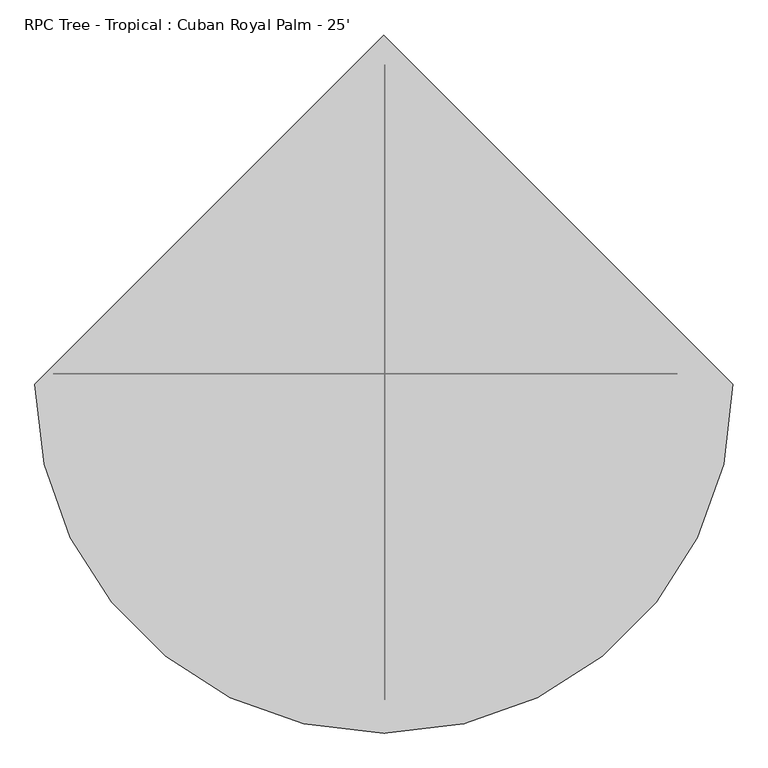
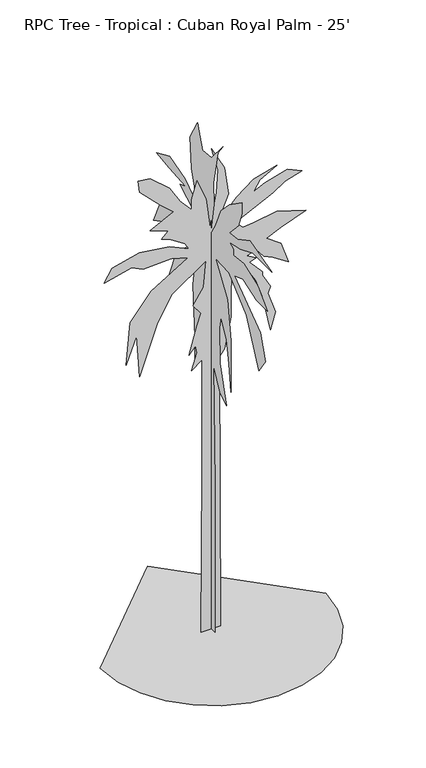
"""IFC4 building model written with IfcOpenShell, lengths in millimetres: geographic element geometry, RPC Tree - Tropical : Cuban Royal Palm - 25'."""

from ifc_helpers import new_model, si_unit, origin, place, context, project, spatial, triangles, source, transform, mapped, element, save


def rpc_tree_tropical_cuban_royal_palm_25_6f0ceb55(model_context):
    return source(origin(), model_context, "Body", "Tessellation", [
        triangles([(-54.3826135, -0.017491, 0.0009437), (-150.0419681, -0.0174994, 0.0009479), (-130.9099418, -0.0179382, 2494.6483109), (-130.9096875, -0.0182426, 4197.3711227), (-283.9640988, -0.0182154, 4082.5885941), (-207.4377743, -0.0182632, 4331.3053894), (-226.5690375, -0.0182829, 4446.0876274), (-322.2291687, -0.0182582, 4331.3053894), (-207.4375199, -0.0183385, 4752.2081863), (-150.0417137, -0.0183718, 4924.3947693), (-264.8328356, -0.0183942, 5077.4551941), (-111.778179, -0.0184419, 5307.0196701), (-73.5143854, -0.0185154, 5708.7968903), (-570.9431663, -0.0184321, 5364.4237244), (-781.3921303, -0.0183579, 5000.9249817), (-1049.2399527, -0.0182128, 4254.775177), (-1087.5024427, -0.0183274, 4905.2686111), (-1240.5575626, -0.0182489, 4503.4916817), (-1183.1638275, -0.0183643, 5134.8336685), (-877.0535151, -0.0184461, 5517.4841492), (-341.3604137, -0.0185277, 5842.7305756), (-590.0744476, -0.0185305, 5919.260788), (-991.8436014, -0.0185095, 5900.10905), (-1164.030039, -0.0185156, 5976.6392624), (-1565.7991928, -0.018481, 5880.9828918), (-1451.0091064, -0.0185202, 6072.2956329), (-1049.2399527, -0.0185549, 6167.9775833), (-609.2056927, -0.0185639, 6110.5735291), (-322.2291687, -0.0185524, 5976.6392624), (-379.6254836, -0.018567, 6072.2956329), (-609.2056927, -0.0185844, 6225.3560577), (-723.9983225, -0.0185862, 6263.6339539), (-628.3394812, -0.0186075, 6359.2903244), (-896.1847601, -0.0186129, 6454.9461136), (-551.8119212, -0.0186587, 6627.1326965), (-743.1295675, -0.0186811, 6799.3192795), (-1049.2399527, -0.0187225, 7105.4395477), (-1068.3711977, -0.0187524, 7277.6261307), (-896.1847601, -0.0187566, 7258.4743927), (-609.2056927, -0.0187246, 7009.7581787), (-456.1505364, -0.0186868, 6761.0413834), (-283.9640988, -0.0186602, 6569.7286423), (-283.9640988, -0.0186875, 6722.7890671), (-207.4375199, -0.0187388, 6990.6320206), (-73.5143854, -0.0186865, 6665.3850128), (-16.1188494, -0.0186069, 6206.2298996), (79.5405301, -0.0187, 6703.6629089), (98.6725473, -0.0187624, 7048.0354935), (3.0131737, -0.0188232, 7411.5348175), (194.3319064, -0.0187666, 7048.0354935), (251.7277126, -0.0186938, 6627.1326965), (79.5405301, -0.018611, 6206.2298996), (366.5190888, -0.0186818, 6531.476326), (615.2330864, -0.0187268, 6722.7890671), (959.6059616, -0.018759, 6818.4454376), (710.8919277, -0.0187242, 6684.5367508), (615.2330864, -0.0186926, 6531.476326), (787.419524, -0.0187138, 6608.0065384), (1112.6611542, -0.0187452, 6703.6629089), (1323.1125526, -0.0187373, 6608.0065384), (1074.3985914, -0.0187127, 6531.476326), (902.2121538, -0.0186847, 6416.6687988), (347.3878438, -0.0186125, 6148.8258453), (462.1779302, -0.018597, 6034.0433167), (615.2330864, -0.0186071, 6053.1694748), (959.6059616, -0.0186324, 6110.5735291), (1380.5089039, -0.0186269, 5976.6392624), (1017.0023129, -0.018587, 5842.7305756), (806.550769, -0.0185607, 5747.074205), (1017.0023129, -0.0185426, 5594.0143616), (1131.7923992, -0.0184894, 5268.7673538), (902.2121538, -0.0185068, 5421.8277786), (768.288279, -0.0185112, 5479.2062531), (615.2330864, -0.0185387, 5670.544574), (615.2330864, -0.0185284, 5613.1405197), (519.5742451, -0.0185174, 5574.8882034), (653.4956491, -0.0185096, 5498.357991), (557.8367715, -0.0184985, 5460.0800949), (749.1570339, -0.0184693, 5249.6411957), (749.1570339, -0.018459, 5192.2371414), (863.9471203, -0.0184264, 4981.7988235), (825.6846302, -0.0184076, 4886.142453), (940.4747166, -0.0183545, 4560.8957359), (863.9471203, -0.0183067, 4312.1792313), (749.1570339, -0.0184009, 4866.990715), (653.4956491, -0.018448, 5153.9848251), (481.3092115, -0.0184918, 5440.9539368), (309.1227739, -0.0184979, 5517.4841492), (289.9915107, -0.0184287, 5134.8336685), (289.9915107, -0.0183534, 4713.9558701), (194.3319064, -0.0182671, 4254.775177), (117.8043192, -0.0182467, 4159.1188065), (136.9360911, -0.0175052, 0.0009354), (-0.003708, 89.5986644, 0.000495), (-0.0037084, 163.6334895, 0.0005082), (-0.003708, 163.6334895, 1826.7789024), (-0.003706, 145.1250443, 4288.4300995), (-0.0037076, 219.1593699, 4177.3813545), (-0.0037057, 404.2456741, 3788.6856033), (-0.0037071, 404.2456741, 4251.4224747), (-0.0037068, 459.7725537, 5028.7883972), (-0.0037083, 385.7367022, 5565.5410995), (-0.0037091, 533.8058619, 5398.9425476), (-0.0037068, 792.9287807, 4862.190136), (-0.0037064, 1089.0671001, 4492.0362762), (-0.0037084, 1311.1695316, 4140.3737297), (-0.0037071, 1052.0491562, 4843.6988228), (-0.0037074, 885.4710245, 5250.8858871), (-0.0037074, 515.2968899, 5621.065036), (-0.003709, 681.8750216, 5584.0318314), (-0.0037073, 903.9799965, 5565.5410995), (-0.0037076, 1107.5760721, 5602.5487244), (-0.0037076, 1459.2413074, 5417.4588593), (-0.0037087, 1274.1542038, 5824.6462143), (-0.0037067, 1070.5581282, 5824.6462143), (-0.0037071, 996.5223129, 6139.3008453), (-0.0037076, 644.859621, 6065.2600159), (-0.0037089, 422.7546461, 6176.3084702), (-0.0037091, 792.9287807, 6379.9146469), (-0.0037059, 644.859621, 6435.4391647), (-0.0037081, 1052.0491562, 6472.4467896), (-0.0037064, 1385.2054195, 6509.4799942), (-0.0037073, 1052.0491562, 6657.5366547), (-0.0037075, 663.368593, 6546.487619), (-0.0037092, 348.7187945, 6324.3907104), (-0.003707, 496.7904977, 6805.6183136), (-0.0037068, 533.8058619, 7268.3296051), (-0.0037076, 348.7187945, 7601.4755493), (-0.0037068, 311.703394, 7490.427095), (-0.0037069, 219.1593699, 7249.8132935), (-0.0037086, -2.9445681, 7268.3296051), (-0.0037062, -299.0821622, 7619.9924423), (-0.0037078, -169.5227376, 7453.4194702), (-0.0037084, -58.4704863, 6916.6673492), (-0.0037085, -76.9791948, 6602.0121368), (-0.003709, 15.5640629, 6083.7763275), (-0.0037058, -113.9968663, 6287.3575058), (-0.0037085, -243.5573174, 6602.0121368), (-0.0037085, -465.6602757, 6824.1096268), (-0.003709, -780.3075308, 7046.2321152), (-0.003709, -780.3075308, 6879.6341446), (-0.0037083, -687.765287, 6639.0453415), (-0.0037091, -465.6602757, 6398.4315399), (-0.0037063, -669.256315, 6416.9228531), (-0.0037092, -983.9036064, 6583.4958252), (-0.0037074, -1539.164772, 6435.4391647), (-0.0037081, -1057.9394217, 6435.4391647), (-0.0037072, -743.2921303, 6305.8738174), (-0.0037083, -465.6602757, 6250.3492996), (-0.0037076, -558.2050993, 6194.8253632), (-0.003708, -558.2050993, 6102.2932205), (-0.0037077, -835.8344467, 6139.3008453), (-0.0037071, -1187.4996094, 6009.735498), (-0.0037064, -1428.1110855, 5769.1216965), (-0.0037087, -1150.4816654, 5769.1216965), (-0.0037066, -798.8165028, 5880.1701508), (-0.0037081, -595.2230069, 5806.1549011), (-0.0037069, -1243.0264526, 5324.9267166), (-0.0037071, -1372.586713, 4954.7475677), (-0.0037067, -1206.0085814, 4714.1337662), (-0.0037072, -891.36129, 5380.4512344), (-0.0037069, -447.1538472, 5769.1216965), (-0.003706, -113.9968663, 5787.6380081), (-0.0037066, -410.1359396, 5324.9267166), (-0.0037068, -502.6781834, 4751.141391), (-0.0037091, -502.6781834, 3955.2841553), (-0.0037069, -447.1538472, 4362.470929), (-0.003708, -391.6269676, 4695.6171638), (-0.0037083, -243.5573174, 4954.7475677), (-0.0037075, -206.5399003, 4769.6579933), (-0.0037065, -225.0485998, 4232.9058723), (-0.0037092, -391.6269676, 3677.6368584), (-0.0037079, -225.0485998, 3788.6856033), (-0.0037085, -58.4704863, 4103.3405251), (-0.0037063, -95.4881577, 2289.4952808), (-0.0037089, -95.4881577, 0.0004619), (-1653.0963352, -49.1291369, 0.0005424), (-1609.512513, -426.8745255, 0.000473), (-1485.3879673, -773.7746447, 0.0004055), (-1290.6616264, -1079.890044, 0.0003423), (-1035.2724913, -1335.2792519, 0.0002854), (-729.1570919, -1530.0055927, 0.0002372), (-382.2594435, -1654.1301384, 0.0001999), (-4.5121786, -1697.7139606, 0.0001756), (373.234849, -1654.1301384, 0.0001668), (720.1324247, -1530.0055927, 0.0001739), (1026.2478968, -1335.2792519, 0.0001953), (1281.6370319, -1079.890044, 0.0002298), (1476.3633728, -773.7746447, 0.000276), (1600.4879185, -426.8745255, 0.0003326), (1644.0717407, -49.1291369, 0.0003983), (-4.5124832, 1599.4541153, 0.0003027)], [[54, 55, 56], [48, 49, 50], [17, 18, 19], [15, 16, 17], [7, 8, 9], [83, 84, 85], [82, 83, 85], [4, 5, 6], [70, 71, 72], [66, 67, 68], [43, 44, 45], [59, 60, 61], [24, 25, 26], [24, 26, 27], [33, 34, 35], [76, 77, 78], [58, 59, 61], [58, 61, 62], [31, 32, 33], [42, 43, 45], [42, 45, 46], [37, 38, 39], [54, 56, 57], [53, 54, 57], [23, 24, 27], [23, 27, 28], [22, 23, 28], [22, 28, 29], [21, 22, 29], [58, 62, 63], [57, 58, 63], [53, 57, 63], [52, 53, 63], [36, 37, 39], [36, 39, 40], [36, 40, 41], [35, 36, 41], [35, 41, 42], [69, 70, 72], [69, 72, 73], [69, 73, 74], [65, 66, 68], [65, 68, 69], [65, 69, 74], [64, 65, 74], [47, 48, 50], [47, 50, 51], [46, 47, 51], [46, 51, 52], [33, 35, 42], [82, 85, 86], [81, 82, 86], [80, 81, 86], [33, 42, 46], [31, 33, 46], [30, 31, 46], [29, 30, 46], [15, 17, 19], [15, 19, 20], [14, 15, 20], [14, 20, 21], [13, 14, 21], [92, 93, 1], [92, 1, 2], [92, 2, 3], [92, 3, 4], [80, 86, 87], [79, 80, 87], [78, 79, 87], [76, 78, 87], [76, 87, 88], [13, 21, 29], [13, 29, 46], [13, 46, 52], [13, 52, 63], [13, 63, 64], [13, 64, 74], [13, 74, 75], [13, 75, 76], [13, 76, 88], [12, 13, 88], [12, 88, 89], [11, 12, 89], [10, 11, 89], [10, 89, 90], [9, 10, 90], [9, 90, 91], [7, 9, 91], [6, 7, 91], [4, 6, 91], [92, 4, 91], [131, 132, 133], [165, 166, 167], [105, 106, 107], [145, 146, 147], [165, 167, 168], [98, 99, 100], [131, 133, 134], [121, 122, 123], [104, 105, 107], [112, 113, 114], [171, 172, 173], [171, 173, 174], [153, 154, 155], [127, 128, 129], [118, 119, 120], [112, 114, 115], [139, 140, 141], [139, 141, 142], [159, 160, 161], [158, 159, 161], [157, 158, 161], [157, 161, 162], [104, 107, 108], [103, 104, 108], [103, 108, 109], [102, 103, 109], [127, 129, 130], [121, 123, 124], [120, 121, 124], [120, 124, 125], [118, 120, 125], [153, 155, 156], [152, 153, 156], [151, 152, 156], [151, 156, 157], [126, 127, 130], [145, 147, 148], [144, 145, 148], [144, 148, 149], [143, 144, 149], [139, 142, 143], [138, 139, 143], [137, 138, 143], [137, 143, 149], [175, 176, 94], [175, 94, 95], [175, 95, 96], [175, 96, 97], [174, 175, 97], [111, 112, 115], [115, 116, 117], [111, 115, 117], [110, 111, 117], [109, 110, 117], [165, 168, 169], [164, 165, 169], [130, 131, 134], [126, 130, 134], [126, 134, 135], [125, 126, 135], [125, 135, 136], [118, 125, 136], [151, 157, 162], [171, 174, 97], [170, 171, 97], [109, 117, 118], [109, 118, 136], [102, 109, 136], [97, 98, 100], [97, 100, 101], [170, 97, 101], [169, 170, 101], [169, 101, 102], [164, 169, 102], [163, 164, 102], [163, 102, 136], [151, 162, 163], [151, 163, 136], [151, 136, 137], [151, 137, 149], [151, 149, 150], [191, 192, 177], [190, 191, 177], [190, 177, 178], [189, 190, 178], [189, 178, 179], [189, 179, 180], [188, 189, 180], [187, 188, 180], [187, 180, 181], [187, 181, 182], [187, 182, 183], [187, 183, 184], [187, 184, 185], [187, 185, 186]], closed=False),
    ])


if __name__ == "__main__":
    model = new_model("IFC4")
    model_context = context("Model", 3, world=origin())
    ifc_project = project(units=[si_unit("LENGTHUNIT", "METRE", prefix="MILLI")], contexts=[model_context])
    site = spatial("IfcSite", under=ifc_project)
    building = spatial("IfcBuilding", under=site)
    placement = place(None, origin())
    rpc_tree_tropical_cuban_royal_palm_25_shape = rpc_tree_tropical_cuban_royal_palm_25_6f0ceb55(model_context)
    element("IfcGeographicElement", 1, ObjectType="RPC Tree - Tropical : Cuban Royal Palm - 25'", at=placement, inside=building, context=model_context, shape_type="MappedRepresentation", body=[
        mapped(rpc_tree_tropical_cuban_royal_palm_25_shape, transform((0.0, 0.0, 0.0), x_axis=(1.0, 0.0, 0.0), y_axis=(0.0, 1.0, 0.0), z_axis=(0.0, 0.0, 1.0))),
    ])
    save(model, "model.ifc")

# Revit data of these elements
# Type "RPC Tree - Tropical : Cuban Royal Palm - 25'"
#   built-in parameter 1005198 = "{2, 15},{39, RPC-16-FVGV-NKG0-7NHH-C000-ST1L-LVER-AU},{1, 0},{1, 0},{2, 35},{1, 8},{5, Color},{1, 0},{1, 0},{3, 0.8},{3, 0.8},{3, 0.8},{1, 8},{7, BBoxMin},{1, 0},{1, 0},{1, 0},{1, 0},{1, 0},{1, 8},{7, BBoxMax},{1, 0},{1, 0},{1, 0},{1, 0},{1, 0},{2, 11},{9, RPCTypeId},{1, 0},{1, 0},{39, RPC-16-FVGV-NKG0-7NHH-C000-ST1L-LVER-AU},{1, 6},{14, RPCPlantHeight},{1, 0},{1, 0},{2, 25},{2, 11},{7, keyword},{1, 0},{1, 0},{72, :Geometry:RPC:Cuban Royal Palm:Roystonea regia (Oreodoxa):palm:tropical.},{2, 11},{8, category},{1, 0},{1, 0},{17, :Trees [Tropical]},{2, 11},{12, LocalizedUID},{1, 0},{1, 0},{16, Cuban Royal Palm},{2, 14},{6, Height},{1, 0},{1, 0},{2, 25},{1, 2},{16, Cast Reflections},{1, 0},{1, 0},{1, 0},{1, 2},{12, Cast Shadows},{1, 0},{1, 0},{1, 1},{1, 2},{9, Lock View},{1, 0},{1, 0},{1, 0},{1, 4},{5, ViewC},{1, 0},{1, 0},{1, 0},{2, 11},{20, AdvancedUIDefinition},{1, 0},{1, 0},{0, },{2, 11},{10, AssetLibID},{1, 0},{1, 0},{36, 4D3F6E72-3F99-4203-98E9-AF80B3C7A7A4},{2, 11},{10, BaseSchema},{1, 0},{1, 0},{9, RPCSchema},{2, 11},{12, ExchangeGUID},{1, 0},{1, 0},{0, },{1, 2},{6, Hidden},{1, 0},{1, 0},{1, 0},{1, 4},{11, RPCCategory},{1, 0},{1, 0},{1, 0},{2, 11},{8, RPCImage},{1, 0},{1, 0},{0, },{1, 4},{13, SchemaVersion},{1, 0},{1, 0},{1, 4},{2, 11},{12, UIDefinition},{1, 0},{1, 0},{0, },{2, 11},{6, UIName},{1, 0},{1, 0},{39, RPC-16-FVGV-NKG0-7NHH-C000-ST1L-LVER-AU},{2, 11},{11, VersionGUID},{1, 0},{1, 0},{9, RPCSchema},{2, 11},{9, assettype},{1, 0},{1, 0},{11, RPCGeometry},{2, 11},{11, description},{1, 0},{1, 0},{0, },{2, 11},{9, localname},{1, 0},{1, 0},{3, RPC},{2, 11},{9, localtype},{1, 0},{1, 0},{3, RPC},{1, 4},{8, revision},{1, 0},{1, 0},{1, 1},{2, 11},{9, thumbnail},{1, 0},{1, 0},{0, },{1, 4},{7, version},{1, 0},{1, 0},{1, 1},{1, 2},{20, RPC_Cast Reflections},{1, 0},{1, 0},{1, 1},{1, 2},{16, RPC_Cast Shadows},{1, 0},{1, 0},{1, 1},{1, 2},{13, RPC_Lock View},{1, 0},{1, 0},{1, 0},{1, 4},{9, RPC_ViewC},{1, 0},{1, 0},{1, 0},{21, assetlibrary_base.fbx},{1, 5},"
#   built-in parameter 1005195 = "RPC-16-FVGV-NKG0-7NHH-C000-ST1L-LVER-AU"
#   Type Comments = "Cuban Royal Palm"
#   Assembly Code = "G2050500"
#   Height = 25' - 0"
#   Plan Symbol = element 419189
#   Default Elevation = 0
